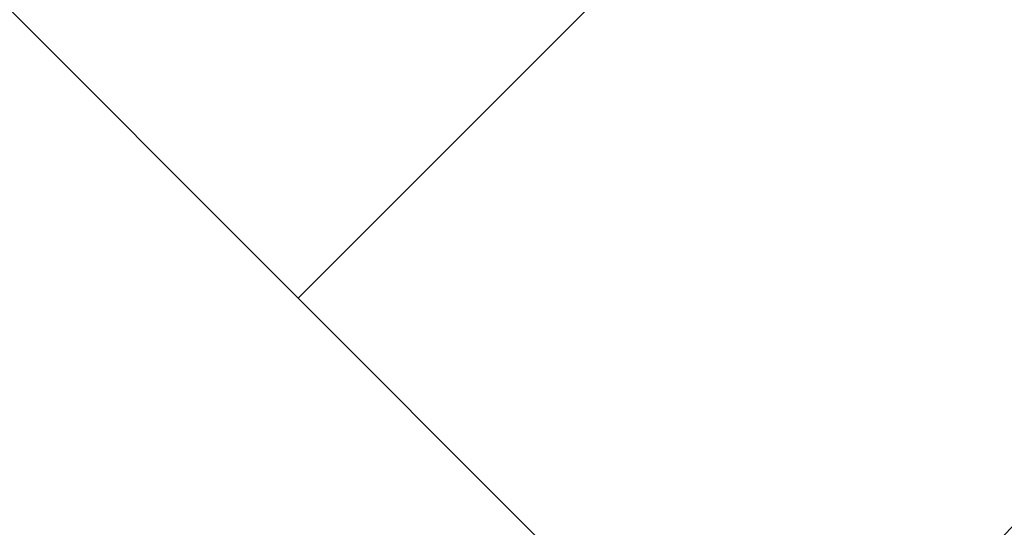
# Model space of a CAD drawing. Units: inches. Extents: x 3590 to 5167, y 65 to 1917.
# Tile 42 of 100: x 5035 to 5065, y 1372 to 1388. Entities that reach past the tile are written whole.
import ezdxf

# ---------------------------------------------------------------- set-up
doc = ezdxf.new("R2010")
doc.units = ezdxf.units.IN
doc.layers.add('A-FLOR-PATT', color=8, linetype='Continuous', lineweight=13)

msp = doc.modelspace()

# ---------------------------------------------------------------- hatches: boundary and pattern name
at = {"layer": 'A-FLOR-PATT', "transparency": 33554687}
h = msp.add_hatch(dxfattribs=at)
h.set_pattern_fill('AR-HBONE', color=256, scale=0.2)
h.set_pattern_definition([(45, (-588.972, 0), (0, 28.73682), [60.96, -20.32]), (135, (-574.604, 14.368), (3e-15, 28.73682), [60.96, -20.32])])
h.paths.add_polyline_path([(5071.274, 1796.999), (4933.274, 1796.999), (4933.274, 1753.999), (4962.774, 1753.999, -0.414214), (4928.774, 1719.999), (4933.274, 1718.999), (4933.274, 1334.999), (5071.274, 1334.999)])
h.paths.add_polyline_path([(4951.78, 1521.077), (4951.715, 1521.04), (4951.563, 1520.895)], flags=16)
h.paths.add_polyline_path([(4952.267, 1521.376), (4952.198, 1521.371), (4952.198, 1521.356)], flags=0)
h.paths.add_polyline_path([(4967.051, 1529.728), (4965.231, 1528.694), (4963.411, 1527.714), (4961.756, 1526.851), (4963.589, 1527.449), (4964.036, 1527.478), (4962.975, 1527.249), (4961.76, 1526.852), (4959.792, 1525.834), (4958.005, 1524.895), (4956.24, 1523.93), (4954.504, 1522.919), (4954.129, 1522.682), (4953.361, 1521.997), (4953.366, 1521.998), (4953.605, 1522.064), (4955.106, 1522.761), (4956.921, 1523.434), (4958.678, 1523.915), (4960.358, 1524.2), (4961.945, 1524.286), (4964.171, 1524.108), (4965.958, 1523.309), (4963.863, 1522.976), (4965.187, 1522.499), (4963.366, 1522.497), (4961.545, 1522.487), (4959.764, 1522.461), (4958.304, 1522.419), (4957.974, 1522.388), (4956.307, 1522.232), (4954.718, 1522.071), (4953.251, 1521.899), (4953.525, 1521.623), (4954.331, 1521.379), (4956.243, 1521.23), (4958.039, 1520.93), (4959.684, 1520.483), (4961.16, 1519.896), (4963.107, 1518.8), (4964.393, 1517.325), (4962.973, 1517.726), (4964.558, 1516.661), (4965.407, 1515.708), (4963.507, 1516.322), (4961.68, 1517.005), (4959.935, 1517.745), (4958.282, 1518.528), (4956.732, 1519.343), (4955.295, 1520.175), (4954.672, 1520.572), (4954.513, 1520.627), (4955.658, 1519.318), (4956.703, 1517.982), (4957.644, 1516.647), (4958.485, 1515.334), (4959.55, 1513.524), (4960.438, 1511.769), (4958.841, 1513.62), (4957.452, 1515.325), (4955.819, 1517.459), (4956.665, 1515.448), (4957.111, 1513.923), (4957.447, 1511.714), (4957.076, 1509.793), (4956.538, 1511.11), (4955.992, 1512.569), (4955.444, 1514.125), (4954.898, 1515.735), (4954.357, 1517.356), (4953.824, 1518.943), (4953.305, 1520.452), (4953.065, 1521.116), (4952.971, 1521.146), (4952.949, 1521.086), (4952.73, 1520.199), (4953.37, 1518.024), (4953.757, 1516.373), (4954.051, 1514.765), (4954.264, 1513.221), (4954.471, 1511.131), (4954.497, 1510.402), (4954.409, 1511.76), (4954.264, 1513.221), (4954.051, 1514.765), (4953.757, 1516.373), (4953.37, 1518.024), (4952.877, 1519.698), (4952.716, 1520.141), (4952.533, 1519.059), (4952.374, 1517.789), (4952.219, 1516.312), (4952.046, 1514.6), (4951.833, 1512.626), (4951.557, 1510.363), (4951.203, 1512.168), (4950.852, 1514.339), (4950.985, 1516.376), (4951.66, 1518.286), (4952.593, 1520.481), (4952.357, 1521.13), (4951.855, 1520.328), (4950.839, 1518.908), (4949.777, 1517.587), (4948.916, 1516.617), (4948.111, 1515.256), (4947.089, 1513.554), (4945.889, 1511.615), (4946.326, 1513.402), (4946.562, 1514.249), (4945.528, 1513.327), (4944.581, 1512.531), (4946.018, 1514.508), (4947.204, 1516.048), (4947.893, 1517.313), (4949.307, 1518.764), (4950.414, 1519.767), (4950.451, 1519.806), (4952.267, 1521.376), (4951.645, 1521.493), (4950.404, 1521.18), (4948.044, 1520.359), (4946.119, 1519.452), (4944.572, 1518.475), (4943.35, 1517.443), (4941.997, 1515.92), (4941.661, 1515.275), (4942.813, 1516.99), (4944.572, 1518.475), (4946.119, 1519.452), (4948.044, 1520.359), (4950.404, 1521.18), (4951.645, 1521.493), (4949.647, 1521.868), (4948.6, 1521.756), (4947.126, 1521.57), (4945.42, 1521.348), (4943.45, 1521.105), (4941.183, 1520.856), (4942.86, 1521.613), (4943.873, 1522.03), (4942.952, 1521.909), (4941.41, 1521.485), (4939.543, 1520.67), (4938.968, 1520.226), (4940.733, 1521.299), (4942.952, 1521.909), (4943.702, 1522.008), (4945.894, 1522.7), (4947.565, 1522.714), (4948.921, 1522.566), (4951.131, 1522.183), (4950.971, 1522.297), (4948.129, 1523.006), (4946.035, 1523.707), (4944.232, 1524.521), (4942.707, 1525.461), (4941.444, 1526.537), (4940.43, 1527.761), (4939.649, 1529.143), (4941.421, 1528.122), (4943.147, 1527.132), (4944.841, 1526.175), (4946.514, 1525.25), (4948.179, 1524.359), (4948.365, 1524.263), (4946.475, 1526.045), (4945.181, 1527.54), (4944.19, 1529.033), (4943.496, 1530.54), (4943.278, 1531.36), (4942.498, 1531.919), (4943.114, 1531.762), (4942.959, 1533.659), (4944.14, 1531.989), (4944.612, 1531.323), (4946.202, 1530.463), (4947.486, 1529.509), (4948.79, 1528.226), (4950.368, 1526.237), (4949.485, 1528.155), (4948.851, 1530.123), (4948.491, 1532.041), (4948.381, 1533.918), (4948.501, 1535.76), (4948.827, 1537.573), (4949.418, 1535.565), (4949.957, 1533.569), (4950.464, 1531.586), (4950.961, 1529.617), (4951.391, 1527.954), (4951.724, 1530.687), (4952.201, 1532.58), (4952.889, 1534.33), (4953.77, 1535.951), (4954.827, 1537.46), (4954.521, 1535.39), (4954.273, 1533.937), (4955.58, 1535.663), (4956.748, 1536.739), (4956.159, 1534.78), (4955.589, 1532.873), (4955.043, 1531.006), (4954.525, 1529.166), (4954.038, 1527.341), (4953.638, 1525.733), (4953.611, 1525.586), (4953.398, 1524.166), (4953.382, 1524.009), (4954.07, 1525.476), (4954.912, 1527.022), (4956.136, 1528.894), (4957.847, 1530.577), (4959.376, 1531.54), (4958.256, 1530.104), (4957.143, 1528.663), (4956.066, 1527.243), (4955.056, 1525.871), (4954.141, 1524.571), (4953.352, 1523.372), (4953.311, 1523.303), (4953.273, 1522.925), (4953.261, 1522.382), (4954.103, 1523.373), (4954.63, 1524.284), (4955.961, 1526.358), (4957.23, 1528.13), (4958.421, 1529.609), (4960.037, 1531.368), (4961.374, 1532.375), (4962.101, 1532.77), (4961.07, 1531.061), (4959.987, 1529.438), (4958.869, 1527.908), (4958.15, 1527.007), (4959.803, 1528.003), (4961.589, 1528.793), (4963.391, 1529.328), (4965.211, 1529.632)], flags=16)
h.paths.add_polyline_path([(4962.944, 1523.182), (4961.107, 1523.422), (4960.392, 1523.362), (4962.35, 1523.331)], flags=0)
h.paths.add_polyline_path([(5049.541, 1584.551), (5049.476, 1584.515), (5049.325, 1584.37)], flags=16)
h.paths.add_polyline_path([(5050.028, 1584.851), (5049.959, 1584.845), (5049.959, 1584.83)], flags=0)
h.paths.add_polyline_path([(5042.333, 1581.949), (5043.88, 1582.926), (5045.806, 1583.833), (5048.165, 1584.654), (5049.406, 1584.967), (5047.408, 1585.342), (5046.361, 1585.231), (5044.888, 1585.044), (5043.181, 1584.822), (5041.211, 1584.579), (5038.944, 1584.33), (5040.622, 1585.087), (5041.634, 1585.504), (5040.713, 1585.383), (5039.171, 1584.959), (5037.304, 1584.144), (5036.729, 1583.7), (5038.494, 1584.773), (5040.713, 1585.383), (5041.463, 1585.482), (5043.655, 1586.174), (5045.326, 1586.188), (5046.682, 1586.04), (5048.893, 1585.657), (5048.732, 1585.771), (5045.891, 1586.48), (5043.796, 1587.181), (5041.994, 1587.996), (5040.468, 1588.935), (5039.205, 1590.011), (5038.191, 1591.235), (5037.41, 1592.617), (5039.182, 1591.596), (5040.909, 1590.607), (5042.602, 1589.649), (5044.275, 1588.724), (5045.94, 1587.833), (5046.126, 1587.738), (5044.237, 1589.519), (5042.942, 1591.015), (5041.952, 1592.508), (5041.257, 1594.014), (5041.039, 1594.834), (5040.26, 1595.393), (5040.875, 1595.237), (5040.721, 1597.133), (5041.901, 1595.463), (5042.373, 1594.798), (5043.963, 1593.938), (5045.247, 1592.983), (5046.552, 1591.701), (5048.129, 1589.712), (5047.247, 1591.63), (5046.613, 1593.597), (5046.252, 1595.515), (5046.142, 1597.392), (5046.262, 1599.234), (5046.588, 1601.047), (5047.179, 1599.039), (5047.718, 1597.043), (5048.225, 1595.06), (5048.722, 1593.091), (5049.152, 1591.429), (5049.485, 1594.161), (5049.962, 1596.054), (5050.65, 1597.804), (5051.532, 1599.425), (5052.589, 1600.934), (5052.283, 1598.864), (5052.034, 1597.411), (5053.341, 1599.137), (5054.509, 1600.213), (5053.92, 1598.254), (5053.35, 1596.348), (5052.805, 1594.48), (5052.286, 1592.64), (5051.799, 1590.815), (5051.4, 1589.207), (5051.373, 1589.06), (5051.159, 1587.64), (5051.143, 1587.483), (5051.831, 1588.95), (5052.673, 1590.496), (5053.898, 1592.368), (5055.608, 1594.051), (5057.137, 1595.014), (5056.017, 1593.578), (5054.904, 1592.137), (5053.828, 1590.717), (5052.817, 1589.345), (5051.902, 1588.046), (5051.113, 1586.846), (5051.072, 1586.777), (5051.034, 1586.399), (5051.022, 1585.856), (5051.864, 1586.847), (5052.391, 1587.758), (5053.723, 1589.832), (5054.991, 1591.604), (5056.182, 1593.083), (5057.798, 1594.842), (5059.135, 1595.849), (5059.863, 1596.244), (5058.831, 1594.535), (5057.749, 1592.912), (5056.63, 1591.382), (5055.912, 1590.482), (5057.564, 1591.477), (5059.35, 1592.267), (5061.152, 1592.802), (5062.972, 1593.106), (5064.812, 1593.203), (5062.992, 1592.169), (5061.172, 1591.188), (5059.518, 1590.325), (5061.35, 1590.924), (5061.797, 1590.952), (5060.737, 1590.723), (5059.521, 1590.326), (5057.553, 1589.308), (5055.766, 1588.369), (5054.002, 1587.404), (5052.265, 1586.393), (5051.891, 1586.156), (5051.122, 1585.471), (5051.127, 1585.472), (5051.366, 1585.538), (5052.867, 1586.235), (5054.682, 1586.908), (5056.439, 1587.389), (5058.12, 1587.675), (5059.706, 1587.76), (5061.933, 1587.583), (5063.719, 1586.783), (5061.624, 1586.45), (5062.949, 1585.973), (5061.127, 1585.971), (5059.307, 1585.961), (5057.525, 1585.935), (5056.065, 1585.893), (5055.735, 1585.862), (5054.068, 1585.707), (5052.479, 1585.546), (5051.012, 1585.373), (5051.286, 1585.097), (5052.092, 1584.853), (5054.004, 1584.704), (5055.8, 1584.404), (5057.446, 1583.958), (5058.921, 1583.37), (5060.868, 1582.274), (5062.154, 1580.799), (5060.734, 1581.2), (5062.32, 1580.135), (5063.168, 1579.182), (5061.269, 1579.796), (5059.441, 1580.479), (5057.696, 1581.219), (5056.043, 1582.003), (5054.493, 1582.817), (5053.057, 1583.649), (5052.433, 1584.047), (5052.274, 1584.101), (5053.42, 1582.793), (5054.464, 1581.457), (5055.405, 1580.121), (5056.247, 1578.809), (5057.311, 1576.998), (5058.199, 1575.244), (5056.602, 1577.094), (5055.213, 1578.799), (5053.58, 1580.933), (5054.427, 1578.922), (5054.872, 1577.397), (5055.208, 1575.189), (5054.838, 1573.267), (5054.299, 1574.584), (5053.754, 1576.043), (5053.206, 1577.599), (5052.659, 1579.209), (5052.118, 1580.83), (5051.585, 1582.417), (5051.066, 1583.927), (5050.826, 1584.59), (5050.733, 1584.62), (5050.711, 1584.561), (5050.491, 1583.673), (5051.131, 1581.498), (5051.518, 1579.847), (5051.813, 1578.24), (5052.026, 1576.695), (5052.233, 1574.605), (5052.258, 1573.876), (5052.17, 1575.234), (5052.026, 1576.695), (5051.813, 1578.24), (5051.518, 1579.847), (5051.131, 1581.498), (5050.638, 1583.172), (5050.477, 1583.615), (5050.294, 1582.533), (5050.136, 1581.263), (5049.981, 1579.786), (5049.807, 1578.074), (5049.594, 1576.1), (5049.318, 1573.837), (5048.965, 1575.642), (5048.613, 1577.813), (5048.747, 1579.85), (5049.421, 1581.76), (5050.354, 1583.955), (5050.118, 1584.604), (5049.616, 1583.802), (5048.6, 1582.382), (5047.538, 1581.061), (5046.677, 1580.091), (5045.872, 1578.73), (5044.85, 1577.028), (5043.651, 1575.089), (5044.087, 1576.877), (5044.324, 1577.723), (5043.289, 1576.801), (5042.342, 1576.005), (5043.779, 1577.982), (5044.966, 1579.522), (5045.655, 1580.787), (5047.068, 1582.239), (5048.175, 1583.241), (5048.213, 1583.28), (5050.028, 1584.851), (5049.406, 1584.967), (5048.165, 1584.654), (5045.806, 1583.833), (5043.88, 1582.926), (5042.333, 1581.949), (5041.111, 1580.917), (5039.758, 1579.394), (5039.423, 1578.749), (5040.575, 1580.464)], flags=16)
h.paths.add_polyline_path([(4954.799, 1533.12), (4954.262, 1532.079), (4953.831, 1530.935), (4953.505, 1529.636), (4953.283, 1528.133), (4953.167, 1526.376), (4953.156, 1524.315), (4953.277, 1521.236), (4952.802, 1521.842), (4951.557, 1521.998), (4950.976, 1521.961), (4952.661, 1521.941), (4952.802, 1521.842), (4953.152, 1523.593), (4953.167, 1526.376), (4953.283, 1528.133), (4953.609, 1530.346), (4954.456, 1532.592)], flags=0)
h.paths.add_polyline_path([(5050.563, 1585.316), (5049.318, 1585.472), (5048.737, 1585.435), (5050.422, 1585.415), (5050.563, 1585.316), (5050.914, 1587.067), (5050.928, 1589.851), (5051.045, 1591.607), (5051.371, 1593.82), (5052.217, 1596.066), (5052.56, 1596.594), (5052.024, 1595.554), (5051.592, 1594.409), (5051.266, 1593.11), (5051.045, 1591.607), (5050.928, 1589.851), (5050.918, 1587.789), (5051.038, 1584.71)], flags=0)
h.paths.add_polyline_path([(5058.153, 1586.836), (5060.111, 1586.805), (5060.705, 1586.656), (5058.868, 1586.896)], flags=0)
h.paths.add_polyline_path([(5049.541, 1430.936), (5049.476, 1430.9), (5049.325, 1430.755)], flags=16)
h.paths.add_polyline_path([(5050.028, 1431.236), (5049.959, 1431.231), (5049.959, 1431.215)], flags=0)
h.paths.add_polyline_path([(5046.588, 1447.432), (5047.179, 1445.425), (5047.718, 1443.429), (5048.225, 1441.446), (5048.722, 1439.476), (5049.152, 1437.814), (5049.485, 1440.546), (5049.962, 1442.439), (5050.65, 1444.189), (5051.532, 1445.811), (5052.589, 1447.319), (5052.283, 1445.249), (5052.034, 1443.796), (5053.341, 1445.522), (5054.509, 1446.598), (5053.92, 1444.64), (5053.35, 1442.733), (5052.805, 1440.865), (5052.286, 1439.025), (5051.799, 1437.201), (5051.4, 1435.592), (5051.373, 1435.445), (5051.159, 1434.025), (5051.143, 1433.868), (5051.831, 1435.335), (5052.673, 1436.881), (5053.898, 1438.753), (5055.608, 1440.436), (5057.137, 1441.4), (5056.017, 1439.963), (5054.904, 1438.522), (5053.828, 1437.102), (5052.817, 1435.73), (5051.902, 1434.431), (5051.113, 1433.231), (5051.072, 1433.162), (5051.034, 1432.784), (5051.022, 1432.242), (5051.864, 1433.232), (5052.391, 1434.143), (5053.723, 1436.217), (5054.991, 1437.989), (5056.182, 1439.468), (5057.798, 1441.227), (5059.135, 1442.235), (5059.863, 1442.629), (5058.831, 1440.921), (5057.749, 1439.298), (5056.63, 1437.767), (5055.912, 1436.867), (5057.564, 1437.863), (5059.35, 1438.652), (5061.152, 1439.187), (5062.972, 1439.491), (5064.812, 1439.588), (5062.992, 1438.554), (5061.172, 1437.573), (5059.518, 1436.71), (5061.35, 1437.309), (5061.797, 1437.337), (5060.737, 1437.108), (5059.521, 1436.711), (5057.553, 1435.693), (5055.766, 1434.754), (5054.002, 1433.789), (5052.265, 1432.778), (5051.891, 1432.541), (5051.122, 1431.856), (5051.127, 1431.857), (5051.366, 1431.923), (5052.867, 1432.62), (5054.682, 1433.293), (5056.439, 1433.775), (5058.12, 1434.06), (5059.706, 1434.145), (5061.933, 1433.968), (5063.719, 1433.168), (5061.624, 1432.835), (5062.949, 1432.358), (5061.127, 1432.357), (5059.307, 1432.346), (5057.525, 1432.32), (5056.065, 1432.278), (5055.735, 1432.248), (5054.068, 1432.092), (5052.479, 1431.931), (5051.012, 1431.759), (5051.286, 1431.482), (5052.092, 1431.238), (5054.004, 1431.089), (5055.8, 1430.789), (5057.446, 1430.343), (5058.921, 1429.755), (5060.868, 1428.66), (5062.154, 1427.185), (5060.734, 1427.585), (5062.32, 1426.52), (5063.168, 1425.567), (5061.269, 1426.181), (5059.441, 1426.865), (5057.696, 1427.604), (5056.043, 1428.388), (5054.493, 1429.202), (5053.057, 1430.034), (5052.433, 1430.432), (5052.274, 1430.487), (5053.42, 1429.178), (5054.464, 1427.842), (5055.405, 1426.506), (5056.247, 1425.194), (5057.311, 1423.383), (5058.199, 1421.629), (5056.602, 1423.479), (5055.213, 1425.184), (5053.58, 1427.318), (5054.427, 1425.307), (5054.872, 1423.782), (5055.208, 1421.574), (5054.838, 1419.652), (5054.299, 1420.97), (5053.754, 1422.428), (5053.206, 1423.984), (5052.659, 1425.595), (5052.118, 1427.215), (5051.585, 1428.802), (5051.066, 1430.312), (5050.826, 1430.975), (5050.733, 1431.005), (5050.711, 1430.946), (5050.491, 1430.058), (5051.131, 1427.883), (5051.518, 1426.232), (5051.813, 1424.625), (5052.026, 1423.081), (5052.233, 1420.991), (5052.258, 1420.261), (5052.17, 1421.619), (5052.026, 1423.081), (5051.813, 1424.625), (5051.518, 1426.232), (5051.131, 1427.883), (5050.638, 1429.558), (5050.477, 1430.001), (5050.294, 1428.918), (5050.136, 1427.648), (5049.981, 1426.171), (5049.807, 1424.459), (5049.594, 1422.485), (5049.318, 1420.222), (5048.965, 1422.028), (5048.613, 1424.199), (5048.747, 1426.235), (5049.421, 1428.146), (5050.354, 1430.34), (5050.118, 1430.989), (5049.616, 1430.187), (5048.6, 1428.768), (5047.538, 1427.446), (5046.677, 1426.477), (5045.872, 1425.116), (5044.85, 1423.413), (5043.651, 1421.474), (5044.087, 1423.262), (5044.324, 1424.109), (5043.289, 1423.186), (5042.342, 1422.391), (5043.779, 1424.368), (5044.966, 1425.907), (5045.655, 1427.173), (5047.068, 1428.624), (5048.175, 1429.627), (5048.213, 1429.666), (5050.028, 1431.236), (5049.406, 1431.353), (5048.165, 1431.039), (5045.806, 1430.218), (5043.88, 1429.311), (5042.333, 1428.334), (5041.111, 1427.302), (5039.758, 1425.779), (5039.423, 1425.134), (5040.575, 1426.849), (5042.333, 1428.334), (5043.88, 1429.311), (5045.806, 1430.218), (5048.165, 1431.039), (5049.406, 1431.353), (5047.408, 1431.727), (5046.361, 1431.616), (5044.888, 1431.429), (5043.181, 1431.207), (5041.211, 1430.964), (5038.944, 1430.715), (5040.622, 1431.472), (5041.634, 1431.89), (5040.713, 1431.769), (5039.171, 1431.345), (5037.304, 1430.53), (5036.729, 1430.085), (5038.494, 1431.158), (5040.713, 1431.769), (5041.463, 1431.867), (5043.655, 1432.559), (5045.326, 1432.573), (5046.682, 1432.425), (5048.893, 1432.042), (5048.732, 1432.156), (5045.891, 1432.865), (5043.796, 1433.566), (5041.994, 1434.381), (5040.468, 1435.321), (5039.205, 1436.396), (5038.191, 1437.62), (5037.41, 1439.002), (5039.182, 1437.982), (5040.909, 1436.992), (5042.602, 1436.034), (5044.275, 1435.109), (5045.94, 1434.218), (5046.126, 1434.123), (5044.237, 1435.904), (5042.942, 1437.4), (5041.952, 1438.893), (5041.257, 1440.399), (5041.039, 1441.219), (5040.26, 1441.778), (5040.875, 1441.622), (5040.721, 1443.518), (5041.901, 1441.848), (5042.373, 1441.183), (5043.963, 1440.323), (5045.247, 1439.369), (5046.552, 1438.086), (5048.129, 1436.097), (5047.247, 1438.015), (5046.613, 1439.982), (5046.252, 1441.901), (5046.142, 1443.778), (5046.262, 1445.619)], flags=16)
h.paths.add_polyline_path([(5052.382, 1444.255), (5051.623, 1442.78), (5052.024, 1441.939), (5052.56, 1442.98)], flags=0)
h.paths.add_polyline_path([(5050.563, 1431.701), (5049.318, 1431.857), (5048.737, 1431.821), (5050.422, 1431.8)], flags=0)
h.paths.add_polyline_path([(5058.153, 1433.221), (5060.111, 1433.19), (5060.705, 1433.041), (5058.868, 1433.281)], flags=0)
h.paths.add_polyline_path([(5049.541, 1352.285), (5049.476, 1352.249), (5049.325, 1352.104)], flags=16)
h.paths.add_polyline_path([(5050.028, 1352.585), (5049.959, 1352.58), (5049.959, 1352.564)], flags=0)
h.paths.add_polyline_path([(5046.588, 1368.781), (5047.179, 1366.774), (5047.718, 1364.778), (5048.225, 1362.795), (5048.722, 1360.825), (5049.152, 1359.163), (5049.485, 1361.896), (5049.962, 1363.789), (5050.65, 1365.538), (5051.532, 1367.16), (5052.589, 1368.669), (5052.283, 1366.598), (5052.034, 1365.145), (5053.341, 1366.871), (5054.509, 1367.947), (5053.92, 1365.989), (5053.35, 1364.082), (5052.805, 1362.214), (5052.286, 1360.374), (5051.799, 1358.55), (5051.4, 1356.942), (5051.373, 1356.794), (5051.159, 1355.374), (5051.143, 1355.218), (5051.831, 1356.684), (5052.673, 1358.23), (5053.898, 1360.102), (5055.608, 1361.786), (5057.137, 1362.749), (5056.017, 1361.313), (5054.904, 1359.872), (5053.828, 1358.452), (5052.817, 1357.079), (5051.902, 1355.78), (5051.113, 1354.581), (5051.072, 1354.512), (5051.034, 1354.133), (5051.022, 1353.591), (5051.864, 1354.581), (5052.391, 1355.492), (5053.723, 1357.566), (5054.991, 1359.338), (5056.182, 1360.817), (5057.798, 1362.577), (5059.135, 1363.584), (5059.863, 1363.979), (5058.831, 1362.27), (5057.749, 1360.647), (5056.63, 1359.117), (5055.912, 1358.216), (5057.564, 1359.212), (5059.35, 1360.001), (5061.152, 1360.536), (5062.972, 1360.841), (5064.812, 1360.937), (5062.992, 1359.903), (5061.172, 1358.923), (5059.518, 1358.059), (5061.35, 1358.658), (5061.797, 1358.687), (5060.737, 1358.458), (5059.521, 1358.061), (5057.553, 1357.043), (5055.766, 1356.103), (5054.002, 1355.138), (5052.265, 1354.127), (5051.891, 1353.89), (5051.122, 1353.206), (5051.127, 1353.206), (5051.366, 1353.272), (5052.867, 1353.969), (5054.682, 1354.643), (5056.439, 1355.124), (5058.12, 1355.409), (5059.706, 1355.495), (5061.933, 1355.317), (5063.719, 1354.518), (5061.624, 1354.184), (5062.949, 1353.708), (5061.127, 1353.706), (5059.307, 1353.695), (5057.525, 1353.669), (5056.065, 1353.627), (5055.735, 1353.597), (5054.068, 1353.441), (5052.479, 1353.28), (5051.012, 1353.108), (5051.286, 1352.831), (5052.092, 1352.587), (5054.004, 1352.439), (5055.8, 1352.138), (5057.446, 1351.692), (5058.921, 1351.104), (5060.868, 1350.009), (5062.154, 1348.534), (5060.734, 1348.935), (5062.32, 1347.869), (5063.168, 1346.916), (5061.269, 1347.53), (5059.441, 1348.214), (5057.696, 1348.954), (5056.043, 1349.737), (5054.493, 1350.551), (5053.057, 1351.383), (5052.433, 1351.781), (5052.274, 1351.836), (5053.42, 1350.527), (5054.464, 1349.191), (5055.405, 1347.855), (5056.247, 1346.543), (5057.311, 1344.733), (5058.199, 1342.978), (5056.602, 1344.828), (5055.213, 1346.534), (5053.58, 1348.667), (5054.427, 1346.656), (5054.872, 1345.132), (5055.208, 1342.923), (5054.838, 1341.002), (5054.299, 1342.319), (5053.754, 1343.778), (5053.206, 1345.334), (5052.659, 1346.944), (5052.118, 1348.564), (5051.585, 1350.151), (5051.066, 1351.661), (5050.826, 1352.324), (5050.733, 1352.355), (5050.711, 1352.295), (5050.491, 1351.408), (5051.131, 1349.232), (5051.518, 1347.581), (5051.813, 1345.974), (5052.026, 1344.43), (5052.233, 1342.34), (5052.258, 1341.61), (5052.17, 1342.969), (5052.026, 1344.43), (5051.813, 1345.974), (5051.518, 1347.581), (5051.131, 1349.232), (5050.638, 1350.907), (5050.477, 1351.35), (5050.294, 1350.267), (5050.136, 1348.997), (5049.981, 1347.52), (5049.807, 1345.809), (5049.594, 1343.835), (5049.318, 1341.571), (5048.965, 1343.377), (5048.613, 1345.548), (5048.747, 1347.585), (5049.421, 1349.495), (5050.354, 1351.689), (5050.118, 1352.339), (5049.616, 1351.536), (5048.6, 1350.117), (5047.538, 1348.795), (5046.677, 1347.826), (5045.872, 1346.465), (5044.85, 1344.763), (5043.651, 1342.824), (5044.087, 1344.611), (5044.324, 1345.458), (5043.289, 1344.535), (5042.342, 1343.74), (5043.779, 1345.717), (5044.966, 1347.256), (5045.655, 1348.522), (5047.068, 1349.973), (5048.175, 1350.976), (5048.213, 1351.015), (5050.028, 1352.585), (5049.406, 1352.702), (5048.165, 1352.388), (5045.806, 1351.567), (5043.88, 1350.661), (5042.333, 1349.683), (5041.111, 1348.651), (5039.758, 1347.128), (5039.423, 1346.483), (5040.575, 1348.198), (5042.333, 1349.683), (5043.88, 1350.661), (5045.806, 1351.567), (5048.165, 1352.388), (5049.406, 1352.702), (5047.408, 1353.076), (5046.361, 1352.965), (5044.888, 1352.779), (5043.181, 1352.556), (5041.211, 1352.313), (5038.944, 1352.065), (5040.622, 1352.821), (5041.634, 1353.239), (5040.713, 1353.118), (5039.171, 1352.694), (5037.304, 1351.879), (5036.729, 1351.434), (5038.494, 1352.508), (5040.713, 1353.118), (5041.463, 1353.216), (5043.655, 1353.909), (5045.326, 1353.923), (5046.682, 1353.774), (5048.893, 1353.391), (5048.732, 1353.506), (5045.891, 1354.214), (5043.796, 1354.915), (5041.994, 1355.73), (5040.468, 1356.67), (5039.205, 1357.746), (5038.191, 1358.969), (5037.41, 1360.352), (5039.182, 1359.331), (5040.909, 1358.341), (5042.602, 1357.383), (5044.275, 1356.458), (5045.94, 1355.567), (5046.126, 1355.472), (5044.237, 1357.253), (5042.942, 1358.749), (5041.952, 1360.242), (5041.257, 1361.748), (5041.039, 1362.568), (5040.26, 1363.128), (5040.875, 1362.971), (5040.721, 1364.867), (5041.901, 1363.197), (5042.373, 1362.532), (5043.963, 1361.672), (5045.247, 1360.718), (5046.552, 1359.435), (5048.129, 1357.446), (5047.247, 1359.364), (5046.613, 1361.331), (5046.252, 1363.25), (5046.142, 1365.127), (5046.262, 1366.969)], flags=16)
h.paths.add_polyline_path([(5052.382, 1365.604), (5051.623, 1364.129), (5052.024, 1363.288), (5052.56, 1364.329)], flags=0)
h.paths.add_polyline_path([(4951.78, 1698.041), (4951.715, 1698.005), (4951.563, 1697.859)], flags=16)
h.paths.add_polyline_path([(4952.267, 1698.341), (4952.198, 1698.335), (4952.198, 1698.32)], flags=0)
h.paths.add_polyline_path([(4957.076, 1686.757), (4956.538, 1688.074), (4955.992, 1689.533), (4955.444, 1691.089), (4954.898, 1692.699), (4954.357, 1694.32), (4953.824, 1695.907), (4953.305, 1697.417), (4953.065, 1698.08), (4952.971, 1698.11), (4952.949, 1698.051), (4952.73, 1697.163), (4953.37, 1694.988), (4953.757, 1693.337), (4954.051, 1691.729), (4954.264, 1690.185), (4954.471, 1688.095), (4954.497, 1687.366), (4954.409, 1688.724), (4954.264, 1690.185), (4954.051, 1691.729), (4953.757, 1693.337), (4953.37, 1694.988), (4952.877, 1696.662), (4952.716, 1697.105), (4952.533, 1696.023), (4952.374, 1694.753), (4952.219, 1693.276), (4952.046, 1691.564), (4951.833, 1689.59), (4951.557, 1687.327), (4951.203, 1689.132), (4950.852, 1691.303), (4950.985, 1693.34), (4951.66, 1695.25), (4952.593, 1697.445), (4952.357, 1698.094), (4951.855, 1697.292), (4950.839, 1695.872), (4949.777, 1694.551), (4948.916, 1693.581), (4948.111, 1692.22), (4947.089, 1690.518), (4945.889, 1688.579), (4946.326, 1690.366), (4946.562, 1691.213), (4945.528, 1690.291), (4944.581, 1689.495), (4946.018, 1691.472), (4947.204, 1693.012), (4947.893, 1694.277), (4949.307, 1695.729), (4950.414, 1696.731), (4950.451, 1696.77), (4952.267, 1698.341), (4951.645, 1698.457), (4950.404, 1698.144), (4948.044, 1697.323), (4946.119, 1696.416), (4944.572, 1695.439), (4943.35, 1694.407), (4941.997, 1692.884), (4941.661, 1692.239), (4942.813, 1693.954), (4944.572, 1695.439), (4946.119, 1696.416), (4948.044, 1697.323), (4950.404, 1698.144), (4951.645, 1698.457), (4949.647, 1698.832), (4948.6, 1698.72), (4947.126, 1698.534), (4945.42, 1698.312), (4943.45, 1698.069), (4941.183, 1697.82), (4942.86, 1698.577), (4943.873, 1698.994), (4942.952, 1698.873), (4941.41, 1698.449), (4939.543, 1697.634), (4938.968, 1697.19), (4940.733, 1698.263), (4942.952, 1698.873), (4943.702, 1698.972), (4945.894, 1699.664), (4947.565, 1699.678), (4948.921, 1699.53), (4951.131, 1699.147), (4950.971, 1699.261), (4948.129, 1699.97), (4946.035, 1700.671), (4944.232, 1701.486), (4942.707, 1702.425), (4941.444, 1703.501), (4940.43, 1704.725), (4939.649, 1706.107), (4941.421, 1705.086), (4943.147, 1704.097), (4944.841, 1703.139), (4946.514, 1702.214), (4948.179, 1701.323), (4948.365, 1701.227), (4946.475, 1703.009), (4945.181, 1704.505), (4944.19, 1705.997), (4943.496, 1707.504), (4943.278, 1708.324), (4942.498, 1708.883), (4943.114, 1708.727), (4942.959, 1710.623), (4944.14, 1708.953), (4944.612, 1708.287), (4946.202, 1707.428), (4947.486, 1706.473), (4948.79, 1705.191), (4950.368, 1703.202), (4949.485, 1705.12), (4948.851, 1707.087), (4948.491, 1709.005), (4948.381, 1710.882), (4948.501, 1712.724), (4948.827, 1714.537), (4949.418, 1712.529), (4949.957, 1710.533), (4950.464, 1708.55), (4950.961, 1706.581), (4951.391, 1704.919), (4951.724, 1707.651), (4952.201, 1709.544), (4952.889, 1711.294), (4953.77, 1712.915), (4954.827, 1714.424), (4954.521, 1712.354), (4954.273, 1710.901), (4955.58, 1712.627), (4956.748, 1713.703), (4956.159, 1711.744), (4955.589, 1709.837), (4955.043, 1707.97), (4954.525, 1706.13), (4954.038, 1704.305), (4953.638, 1702.697), (4953.611, 1702.55), (4953.398, 1701.13), (4953.382, 1700.973), (4954.07, 1702.44), (4954.912, 1703.986), (4956.136, 1705.858), (4957.847, 1707.541), (4959.376, 1708.504), (4958.256, 1707.068), (4957.143, 1705.627), (4956.066, 1704.207), (4955.056, 1702.835), (4954.141, 1701.536), (4953.352, 1700.336), (4953.311, 1700.267), (4953.273, 1699.889), (4953.261, 1699.346), (4954.103, 1700.337), (4954.63, 1701.248), (4955.961, 1703.322), (4957.23, 1705.094), (4958.421, 1706.573), (4960.037, 1708.332), (4961.374, 1709.339), (4962.101, 1709.734), (4961.07, 1708.025), (4959.987, 1706.402), (4958.869, 1704.872), (4958.15, 1703.972), (4959.803, 1704.967), (4961.589, 1705.757), (4963.391, 1706.292), (4965.211, 1706.596), (4967.051, 1706.692), (4965.231, 1705.659), (4963.411, 1704.678), (4961.756, 1703.815), (4963.589, 1704.413), (4964.036, 1704.442), (4962.975, 1704.213), (4961.76, 1703.816), (4959.792, 1702.798), (4958.005, 1701.859), (4956.24, 1700.894), (4954.504, 1699.883), (4954.129, 1699.646), (4953.361, 1698.961), (4953.366, 1698.962), (4953.605, 1699.028), (4955.106, 1699.725), (4956.921, 1700.398), (4958.678, 1700.879), (4960.358, 1701.164), (4961.945, 1701.25), (4964.171, 1701.073), (4965.958, 1700.273), (4963.863, 1699.94), (4965.187, 1699.463), (4963.366, 1699.461), (4961.545, 1699.451), (4959.764, 1699.425), (4958.304, 1699.383), (4957.974, 1699.352), (4956.307, 1699.197), (4954.718, 1699.036), (4953.251, 1698.863), (4953.525, 1698.587), (4954.331, 1698.343), (4956.243, 1698.194), (4958.039, 1697.894), (4959.684, 1697.447), (4961.16, 1696.86), (4963.107, 1695.764), (4964.393, 1694.289), (4962.973, 1694.69), (4964.558, 1693.625), (4965.407, 1692.672), (4963.507, 1693.286), (4961.68, 1693.969), (4959.935, 1694.709), (4958.282, 1695.492), (4956.732, 1696.307), (4955.295, 1697.139), (4954.672, 1697.536), (4954.513, 1697.591), (4955.658, 1696.282), (4956.703, 1694.946), (4957.644, 1693.611), (4958.485, 1692.298), (4959.55, 1690.488), (4960.438, 1688.733), (4958.841, 1690.584), (4957.452, 1692.289), (4955.819, 1694.423), (4956.665, 1692.412), (4957.111, 1690.887), (4957.447, 1688.678)], flags=16)
h.paths.add_polyline_path([(5050.563, 1353.05), (5049.318, 1353.207), (5048.737, 1353.17), (5050.422, 1353.15)], flags=0)
h.paths.add_polyline_path([(4951.78, 1351.486), (4951.715, 1351.45), (4951.563, 1351.305)], flags=16)
h.paths.add_polyline_path([(4952.267, 1351.786), (4952.198, 1351.78), (4952.198, 1351.765)], flags=0)
h.paths.add_polyline_path([(4954.827, 1367.869), (4954.521, 1365.799), (4954.273, 1364.346), (4955.58, 1366.072), (4956.748, 1367.148), (4956.159, 1365.19), (4955.589, 1363.283), (4955.043, 1361.415), (4954.525, 1359.575), (4954.038, 1357.751), (4953.638, 1356.142), (4953.611, 1355.995), (4953.398, 1354.575), (4953.382, 1354.418), (4954.07, 1355.885), (4954.912, 1357.431), (4956.136, 1359.303), (4957.847, 1360.986), (4959.376, 1361.95), (4958.256, 1360.513), (4957.143, 1359.072), (4956.066, 1357.652), (4955.056, 1356.28), (4954.141, 1354.981), (4953.352, 1353.781), (4953.311, 1353.712), (4953.273, 1353.334), (4953.261, 1352.792), (4954.103, 1353.782), (4954.63, 1354.693), (4955.961, 1356.767), (4957.23, 1358.539), (4958.421, 1360.018), (4960.037, 1361.777), (4961.374, 1362.785), (4962.101, 1363.179), (4961.07, 1361.471), (4959.987, 1359.848), (4958.869, 1358.317), (4958.15, 1357.417), (4959.803, 1358.413), (4961.589, 1359.202), (4963.391, 1359.737), (4965.211, 1360.041), (4967.051, 1360.138), (4965.231, 1359.104), (4963.411, 1358.123), (4961.756, 1357.26), (4963.589, 1357.859), (4964.036, 1357.887), (4962.975, 1357.658), (4961.76, 1357.261), (4959.792, 1356.243), (4958.005, 1355.304), (4956.24, 1354.339), (4954.504, 1353.328), (4954.129, 1353.091), (4953.361, 1352.406), (4953.366, 1352.407), (4953.605, 1352.473), (4955.106, 1353.17), (4956.921, 1353.843), (4958.678, 1354.325), (4960.358, 1354.61), (4961.945, 1354.695), (4964.171, 1354.518), (4965.958, 1353.718), (4963.863, 1353.385), (4965.187, 1352.908), (4963.366, 1352.907), (4961.545, 1352.896), (4959.764, 1352.87), (4958.304, 1352.828), (4957.974, 1352.798), (4956.307, 1352.642), (4954.718, 1352.481), (4953.251, 1352.309), (4953.525, 1352.032), (4954.331, 1351.788), (4956.243, 1351.639), (4958.039, 1351.339), (4959.684, 1350.893), (4961.16, 1350.305), (4963.107, 1349.21), (4964.393, 1347.735), (4962.973, 1348.135), (4964.558, 1347.07), (4965.407, 1346.117), (4963.507, 1346.731), (4961.68, 1347.414), (4959.935, 1348.154), (4958.282, 1348.938), (4956.732, 1349.752), (4955.295, 1350.584), (4954.672, 1350.982), (4954.513, 1351.036), (4955.658, 1349.728), (4956.703, 1348.392), (4957.644, 1347.056), (4958.485, 1345.744), (4959.55, 1343.933), (4960.438, 1342.179), (4958.841, 1344.029), (4957.452, 1345.734), (4955.819, 1347.868), (4956.665, 1345.857), (4957.111, 1344.332), (4957.447, 1342.124), (4957.076, 1340.202), (4956.538, 1341.52), (4955.992, 1342.978), (4955.444, 1344.534), (4954.898, 1346.145), (4954.357, 1347.765), (4953.824, 1349.352), (4953.305, 1350.862), (4953.065, 1351.525), (4952.971, 1351.555), (4952.949, 1351.496), (4952.73, 1350.608), (4953.37, 1348.433), (4953.757, 1346.782), (4954.051, 1345.175), (4954.264, 1343.631), (4954.471, 1341.541), (4954.497, 1340.811), (4954.409, 1342.169), (4954.264, 1343.631), (4954.051, 1345.175), (4953.757, 1346.782), (4953.37, 1348.433), (4952.877, 1350.108), (4952.716, 1350.551), (4952.533, 1349.468), (4952.374, 1348.198), (4952.219, 1346.721), (4952.046, 1345.009), (4951.833, 1343.035), (4951.557, 1340.772), (4951.203, 1342.578), (4950.852, 1344.749), (4950.985, 1346.785), (4951.66, 1348.696), (4952.593, 1350.89), (4952.357, 1351.539), (4951.855, 1350.737), (4950.839, 1349.318), (4949.777, 1347.996), (4948.916, 1347.027), (4948.111, 1345.665), (4947.089, 1343.963), (4945.889, 1342.024), (4946.326, 1343.812), (4946.562, 1344.659), (4945.528, 1343.736), (4944.581, 1342.941), (4946.018, 1344.918), (4947.204, 1346.457), (4947.893, 1347.723), (4949.307, 1349.174), (4950.414, 1350.177), (4950.451, 1350.216), (4952.267, 1351.786), (4951.645, 1351.903), (4950.404, 1351.589), (4948.044, 1350.768), (4946.119, 1349.861), (4944.572, 1348.884), (4943.35, 1347.852), (4941.997, 1346.329), (4941.661, 1345.684), (4942.813, 1347.399), (4944.572, 1348.884), (4946.119, 1349.861), (4948.044, 1350.768), (4950.404, 1351.589), (4951.645, 1351.903), (4949.647, 1352.277), (4948.6, 1352.166), (4947.126, 1351.979), (4945.42, 1351.757), (4943.45, 1351.514), (4941.183, 1351.265), (4942.86, 1352.022), (4943.873, 1352.44), (4942.952, 1352.319), (4941.41, 1351.895), (4939.543, 1351.08), (4938.968, 1350.635), (4940.733, 1351.708), (4942.952, 1352.319), (4943.702, 1352.417), (4945.894, 1353.109), (4947.565, 1353.123), (4948.921, 1352.975), (4951.131, 1352.592), (4950.971, 1352.706), (4948.129, 1353.415), (4946.035, 1354.116), (4944.232, 1354.931), (4942.707, 1355.871), (4941.444, 1356.946), (4940.43, 1358.17), (4939.649, 1359.552), (4941.421, 1358.532), (4943.147, 1357.542), (4944.841, 1356.584), (4946.514, 1355.659), (4948.179, 1354.768), (4948.365, 1354.673), (4946.475, 1356.454), (4945.181, 1357.95), (4944.19, 1359.443), (4943.496, 1360.949), (4943.278, 1361.769), (4942.498, 1362.328), (4943.114, 1362.172), (4942.959, 1364.068), (4944.14, 1362.398), (4944.612, 1361.733), (4946.202, 1360.873), (4947.486, 1359.919), (4948.79, 1358.636), (4950.368, 1356.647), (4949.485, 1358.565), (4948.851, 1360.532), (4948.491, 1362.451), (4948.381, 1364.328), (4948.501, 1366.169), (4948.827, 1367.982), (4949.418, 1365.975), (4949.957, 1363.979), (4950.464, 1361.995), (4950.961, 1360.026), (4951.391, 1358.364), (4951.724, 1361.096), (4952.201, 1362.989), (4952.889, 1364.739), (4953.77, 1366.361)], flags=16)
h.paths.add_polyline_path([(4954.799, 1363.53), (4954.262, 1362.489), (4953.831, 1361.344), (4953.505, 1360.045), (4953.283, 1358.543), (4953.167, 1356.786), (4953.156, 1354.724), (4953.277, 1351.646), (4952.802, 1352.251), (4951.557, 1352.407), (4950.976, 1352.371), (4952.661, 1352.35), (4952.802, 1352.251), (4953.152, 1354.002), (4953.167, 1356.786), (4953.283, 1358.543), (4953.609, 1360.755), (4954.456, 1363.001)], flags=0)
h.paths.add_polyline_path([(4952.802, 1698.806), (4951.557, 1698.962), (4950.976, 1698.925), (4952.661, 1698.905), (4952.802, 1698.806), (4953.152, 1700.557), (4953.167, 1703.34), (4953.283, 1705.097), (4953.609, 1707.31), (4954.456, 1709.556), (4954.799, 1710.084), (4954.262, 1709.043), (4953.831, 1707.899), (4953.505, 1706.6), (4953.283, 1705.097), (4953.167, 1703.34), (4953.156, 1701.279), (4953.277, 1698.2)], flags=0)
h.paths.add_polyline_path([(4962.944, 1700.146), (4961.107, 1700.386), (4960.392, 1700.326), (4962.35, 1700.295)], flags=0)
h.paths.add_polyline_path([(5058.153, 1354.57), (5060.111, 1354.539), (5060.705, 1354.391), (5058.868, 1354.631)], flags=0)
h.paths.add_polyline_path([(4962.944, 1353.591), (4961.107, 1353.831), (4960.392, 1353.771), (4962.35, 1353.74)], flags=0)
h.paths.add_polyline_path([(5049.541, 1778.72), (5049.476, 1778.684), (5049.325, 1778.539)], flags=16)
h.paths.add_polyline_path([(5050.028, 1779.02), (5049.959, 1779.014), (5049.959, 1778.999)], flags=0)
h.paths.add_polyline_path([(5052.258, 1768.045), (5052.17, 1769.403), (5052.026, 1770.864), (5051.813, 1772.409), (5051.518, 1774.016), (5051.131, 1775.667), (5050.638, 1777.341), (5050.477, 1777.784), (5050.294, 1776.702), (5050.136, 1775.432), (5049.981, 1773.955), (5049.807, 1772.243), (5049.594, 1770.269), (5049.318, 1768.006), (5048.965, 1769.811), (5048.613, 1771.982), (5048.747, 1774.019), (5049.421, 1775.929), (5050.354, 1778.124), (5050.118, 1778.773), (5049.616, 1777.971), (5048.6, 1776.551), (5047.538, 1775.23), (5046.677, 1774.26), (5045.872, 1772.899), (5044.85, 1771.197), (5043.651, 1769.258), (5044.087, 1771.046), (5044.324, 1771.892), (5043.289, 1770.97), (5042.342, 1770.174), (5043.779, 1772.151), (5044.966, 1773.691), (5045.655, 1774.956), (5047.068, 1776.408), (5048.175, 1777.41), (5048.213, 1777.449), (5050.028, 1779.02), (5049.406, 1779.136), (5048.165, 1778.823), (5045.806, 1778.002), (5043.88, 1777.095), (5042.333, 1776.118), (5041.111, 1775.086), (5039.758, 1773.563), (5039.423, 1772.918), (5040.575, 1774.633), (5042.333, 1776.118), (5043.88, 1777.095), (5045.806, 1778.002), (5048.165, 1778.823), (5049.406, 1779.136), (5047.408, 1779.511), (5046.361, 1779.4), (5044.888, 1779.213), (5043.181, 1778.991), (5041.211, 1778.748), (5038.944, 1778.499), (5040.622, 1779.256), (5041.634, 1779.673), (5040.713, 1779.552), (5039.171, 1779.128), (5037.304, 1778.313), (5036.729, 1777.869), (5038.494, 1778.942), (5040.713, 1779.552), (5041.463, 1779.651), (5043.655, 1780.343), (5045.326, 1780.357), (5046.682, 1780.209), (5048.893, 1779.826), (5048.732, 1779.94), (5045.891, 1780.649), (5043.796, 1781.35), (5041.994, 1782.165), (5040.468, 1783.104), (5039.205, 1784.18), (5038.191, 1785.404), (5037.41, 1786.786), (5039.182, 1785.765), (5040.909, 1784.776), (5042.602, 1783.818), (5044.275, 1782.893), (5045.94, 1782.002), (5046.126, 1781.907), (5044.237, 1783.688), (5042.942, 1785.184), (5041.952, 1786.677), (5041.257, 1788.183), (5041.039, 1789.003), (5040.26, 1789.562), (5040.875, 1789.406), (5040.721, 1791.302), (5041.901, 1789.632), (5042.373, 1788.967), (5043.963, 1788.107), (5045.247, 1787.152), (5046.552, 1785.87), (5048.129, 1783.881), (5047.247, 1785.799), (5046.613, 1787.766), (5046.252, 1789.684), (5046.142, 1791.561), (5046.262, 1793.403), (5046.588, 1795.216), (5047.179, 1793.208), (5047.718, 1791.213), (5048.225, 1789.229), (5048.722, 1787.26), (5049.152, 1785.598), (5049.485, 1788.33), (5049.962, 1790.223), (5050.65, 1791.973), (5051.532, 1793.594), (5052.589, 1795.103), (5052.283, 1793.033), (5052.034, 1791.58), (5053.341, 1793.306), (5054.509, 1794.382), (5053.92, 1792.423), (5053.35, 1790.517), (5052.805, 1788.649), (5052.286, 1786.809), (5051.799, 1784.984), (5051.4, 1783.376), (5051.373, 1783.229), (5051.159, 1781.809), (5051.143, 1781.652), (5051.831, 1783.119), (5052.673, 1784.665), (5053.898, 1786.537), (5055.608, 1788.22), (5057.137, 1789.183), (5056.017, 1787.747), (5054.904, 1786.306), (5053.828, 1784.886), (5052.817, 1783.514), (5051.902, 1782.215), (5051.113, 1781.015), (5051.072, 1780.946), (5051.034, 1780.568), (5051.022, 1780.025), (5051.864, 1781.016), (5052.391, 1781.927), (5053.723, 1784.001), (5054.991, 1785.773), (5056.182, 1787.252), (5057.798, 1789.011), (5059.135, 1790.018), (5059.863, 1790.413), (5058.831, 1788.704), (5057.749, 1787.081), (5056.63, 1785.551), (5055.912, 1784.651), (5057.564, 1785.646), (5059.35, 1786.436), (5061.152, 1786.971), (5062.972, 1787.275), (5064.812, 1787.372), (5062.992, 1786.338), (5061.172, 1785.357), (5059.518, 1784.494), (5061.35, 1785.093), (5061.797, 1785.121), (5060.737, 1784.892), (5059.521, 1784.495), (5057.553, 1783.477), (5055.766, 1782.538), (5054.002, 1781.573), (5052.265, 1780.562), (5051.891, 1780.325), (5051.122, 1779.64), (5051.127, 1779.641), (5051.366, 1779.707), (5052.867, 1780.404), (5054.682, 1781.077), (5056.439, 1781.558), (5058.12, 1781.844), (5059.706, 1781.929), (5061.933, 1781.752), (5063.719, 1780.952), (5061.624, 1780.619), (5062.949, 1780.142), (5061.127, 1780.14), (5059.307, 1780.13), (5057.525, 1780.104), (5056.065, 1780.062), (5055.735, 1780.031), (5054.068, 1779.876), (5052.479, 1779.715), (5051.012, 1779.542), (5051.286, 1779.266), (5052.092, 1779.022), (5054.004, 1778.873), (5055.8, 1778.573), (5057.446, 1778.127), (5058.921, 1777.539), (5060.868, 1776.443), (5062.154, 1774.968), (5060.734, 1775.369), (5062.32, 1774.304), (5063.168, 1773.351), (5061.269, 1773.965), (5059.441, 1774.648), (5057.696, 1775.388), (5056.043, 1776.172), (5054.493, 1776.986), (5053.057, 1777.818), (5052.433, 1778.216), (5052.274, 1778.27), (5053.42, 1776.962), (5054.464, 1775.626), (5055.405, 1774.29), (5056.247, 1772.978), (5057.311, 1771.167), (5058.199, 1769.413), (5056.602, 1771.263), (5055.213, 1772.968), (5053.58, 1775.102), (5054.427, 1773.091), (5054.872, 1771.566), (5055.208, 1769.358), (5054.838, 1767.436), (5054.299, 1768.753), (5053.754, 1770.212), (5053.206, 1771.768), (5052.659, 1773.378), (5052.118, 1774.999), (5051.585, 1776.586), (5051.066, 1778.096), (5050.826, 1778.759), (5050.733, 1778.789), (5050.711, 1778.73), (5050.491, 1777.842), (5051.131, 1775.667), (5051.518, 1774.016), (5051.813, 1772.409), (5052.026, 1770.864), (5052.233, 1768.774)], flags=16)
h.paths.add_polyline_path([(5050.563, 1779.485), (5049.318, 1779.641), (5048.737, 1779.604), (5050.422, 1779.584), (5050.563, 1779.485), (5050.914, 1781.236), (5050.928, 1784.02), (5051.045, 1785.776), (5051.371, 1787.989), (5052.217, 1790.235), (5052.56, 1790.763), (5052.024, 1789.723), (5051.592, 1788.578), (5051.266, 1787.279), (5051.045, 1785.776), (5050.928, 1784.02), (5050.918, 1781.958), (5051.038, 1778.879)], flags=0)
h.paths.add_polyline_path([(5058.153, 1781.005), (5060.111, 1780.974), (5060.705, 1780.825), (5058.868, 1781.065)], flags=0)

doc.saveas('drawing.dxf')
